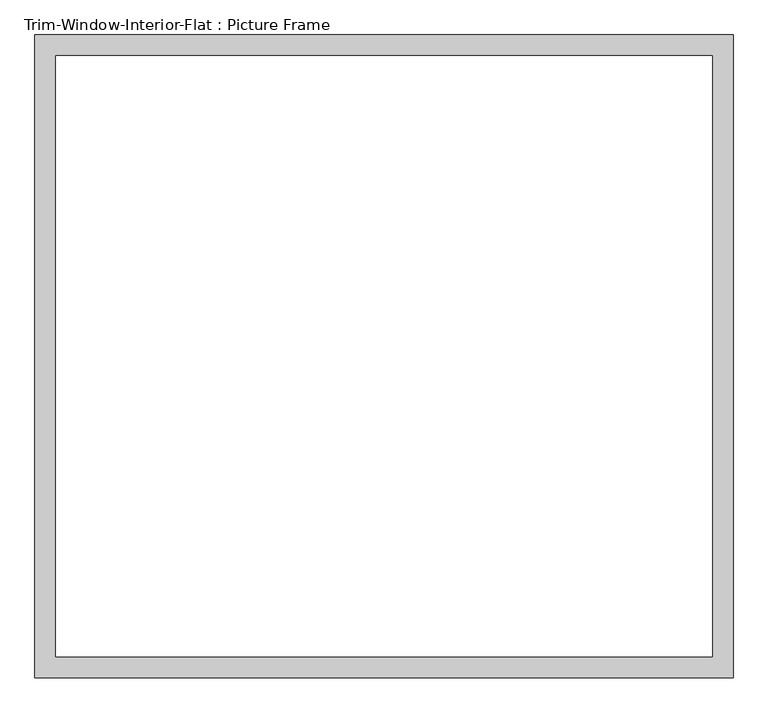
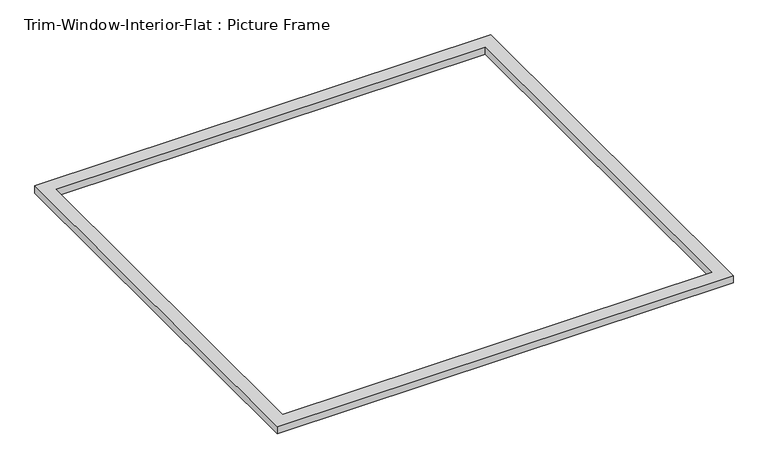
"""IFC4 building model written with IfcOpenShell, lengths in millimetres: proxy geometry, Trim-Window-Interior-Flat : Picture Frame."""

from ifc_helpers import new_model, si_unit, origin, origin_with_axes, place, context, project, spatial, polyline, outline, extrude, source, transform, mapped, element, save


def trim_window_interior_flat_picture_frame_67c405d8(model_context):
    return source(origin(), model_context, "Body", "SweptSolid", [
        extrude(outline(polyline([(958.85, -44.45), (-958.85, -44.45), (-958.85, 1720.85), (958.85, 1720.85), (958.85, -44.45)]), holes=[polyline([(901.7, 12.7), (901.7, 1663.7), (-901.7, 1663.7), (-901.7, 12.7), (901.7, 12.7)])]), origin_with_axes(), (0.0, 0.0, 1.0), 31.75),
    ])


if __name__ == "__main__":
    model = new_model("IFC4")
    model_context = context("Model", 3, world=origin())
    ifc_project = project(units=[si_unit("LENGTHUNIT", "METRE", prefix="MILLI")], contexts=[model_context])
    site = spatial("IfcSite", under=ifc_project)
    building = spatial("IfcBuilding", under=site)
    placement = place(None, origin())
    trim_window_interior_flat_picture_frame_shape = trim_window_interior_flat_picture_frame_67c405d8(model_context)
    element("IfcBuildingElementProxy", 1, Name="Trim-Window-Interior-Flat : Picture Frame", ObjectType="Trim-Window-Interior-Flat : Picture Frame", at=placement, inside=building, context=model_context, shape_type="MappedRepresentation", body=[
        mapped(trim_window_interior_flat_picture_frame_shape, transform((0.0, 0.0, 0.0), x_axis=(1.0, 0.0, 0.0), y_axis=(0.0, 1.0, 0.0), z_axis=(0.0, 0.0, 1.0))),
    ])
    save(model, "model.ifc")

# Revit data of these elements
# Type "Trim-Window-Interior-Flat : Picture Frame"
#   Trim Thickness_Picture Frame = 0' - 1 1/4"
#   Trim Width = 0' - 2 1/4"
#   Trim Thickness_with Sill = 0' - 0 3/4"
#   Sill Thickness = 0' - 1 1/4"
#   Opening Width [instance default] = 2' - 0"
#   Opening Height [instance default] = 3' - 0"
#   Default Elevation = 4' - 0"
#   Sill = no
#   Picture Frame = yes
#   Trim Material [instance default] = none
# Element 1 (IfcBuildingElementProxy, "Trim-Window-Interior-Flat : Picture Frame")
#   Opening Width = 6' - 0"
#   Opening Height = 5' - 6"
#   Trim Material = Wood - Stained
#   Materials on its faces: "Wood - Stained"
# Materials
#   "Wood - Stained": class "Wood", colour RGB 224 178 126, transparency 0, Cost = 0
